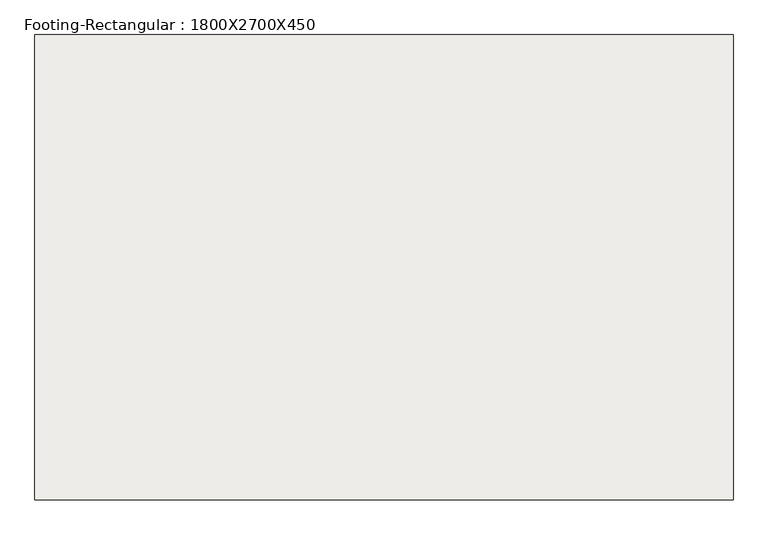
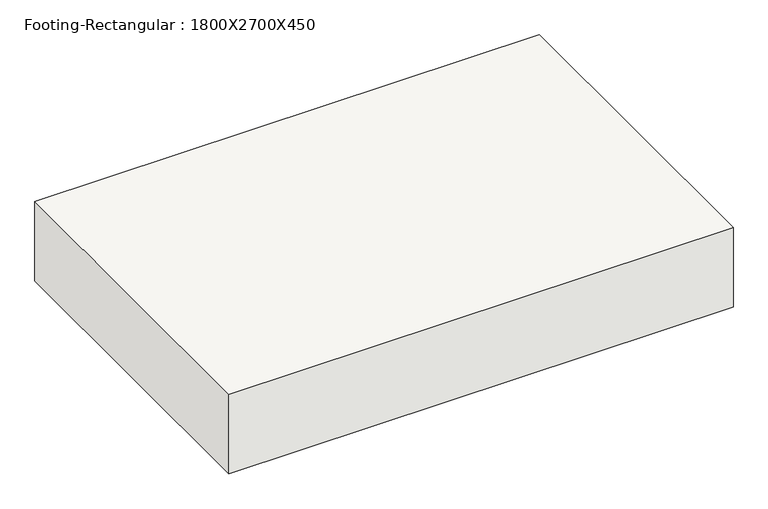
"""IFC4 building model written with IfcOpenShell, lengths in millimetres: slab geometry, Footing-Rectangular : 1800X2700X450."""

from ifc_helpers import new_model, si_unit, frame, origin, place, context, project, spatial, polyline, outline, extrude, source, transform, mapped, element, save


def footing_rectangular_1800x2700x450_79bb3453(model_context):
    return source(origin(), model_context, "Body", "SweptSolid", [
        extrude(outline(polyline([(1350.0, 900.0), (1350.0, -900.0), (-1350.0, -900.0), (-1350.0, 900.0), (1350.0, 900.0)])), frame((0.0, 0.0, -450.0), z_axis=(0.0, 0.0, 1.0), x_axis=(1.0, 0.0, 0.0)), (0.0, 0.0, 1.0), 450.0),
    ])


if __name__ == "__main__":
    model = new_model("IFC4")
    model_context = context("Model", 3, world=origin())
    ifc_project = project(units=[si_unit("LENGTHUNIT", "METRE", prefix="MILLI")], contexts=[model_context])
    site = spatial("IfcSite", under=ifc_project)
    building = spatial("IfcBuilding", under=site)
    placement = place(None, origin())
    footing_rectangular_1800x2700x450_shape = footing_rectangular_1800x2700x450_79bb3453(model_context)
    element("IfcSlab", 1, ObjectType="Footing-Rectangular : 1800X2700X450", at=placement, inside=building, context=model_context, shape_type="MappedRepresentation", body=[
        mapped(footing_rectangular_1800x2700x450_shape, transform((0.0, 0.0, 0.0), x_axis=(1.0, 0.0, 0.0), y_axis=(0.0, 1.0, 0.0), z_axis=(0.0, 0.0, 1.0))),
    ])
    save(model, "model.ifc")

# Revit data of these elements
# Type "Footing-Rectangular : 1800X2700X450"
#   Width = 8' - 10.29921"
#   Length = 5' - 10.86614"
#   Foundation Thickness = 1' - 5.71654"
#   Structural Material [instance default] = Concrete - Cast-in-Place Concrete
#   Assembly Code = ""
# Element 1 (IfcSlab, "Footing-Rectangular : 1800X2700X450")
#   Materials on its faces: "Concrete - Cast-in-Place Concrete"
# Materials
#   "Concrete - Cast-in-Place Concrete": class "Concrete", colour RGB 192 192 192, transparency 0, Cost = 0
